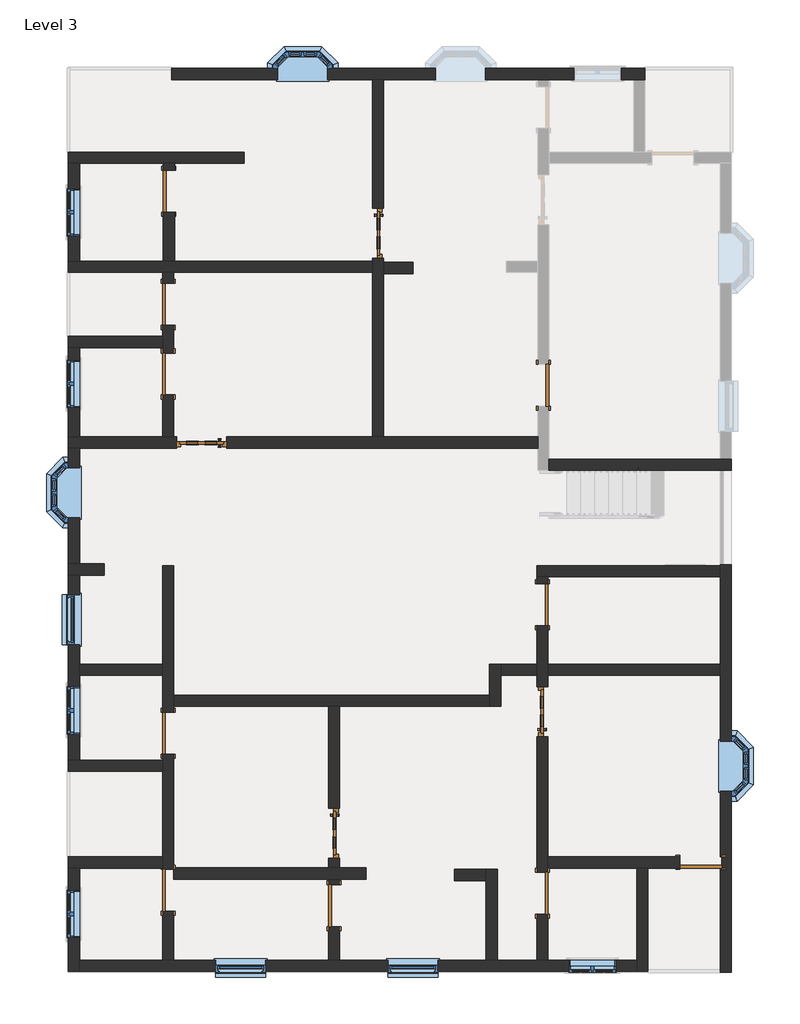
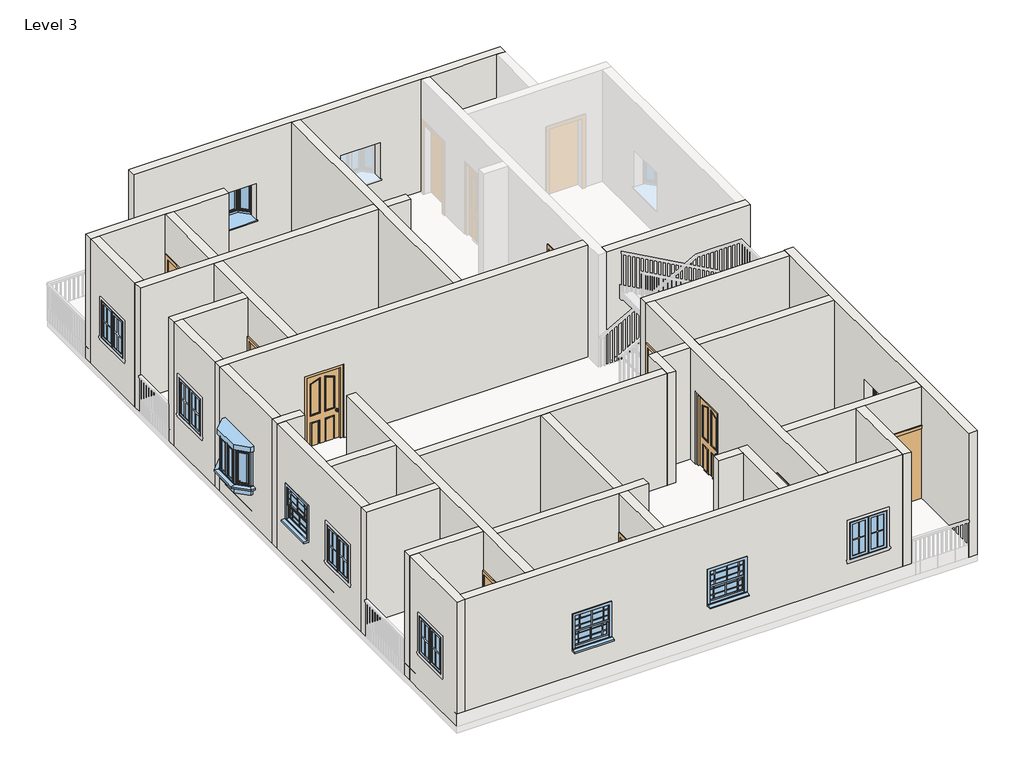
# One storey, part 1 of 4: 34 walls, 14 doors, 11 windows.
"""IFC4 building model written with IfcOpenShell, lengths in millimetres."""

from ifc_helpers import new_model, si_unit, frame, origin, place, context, project, spatial, polyline, outline, extrude, faceted_brep, transform, mapped, element, save
from components import doors_extsgl_12_910x2110mm_9a09825e, door_fadea3f2, door_53b1b562, window_910x910mm_67ef725a, window_c29befe5, windows_sash_w_bars_1_910x910mm_b688f793

model = new_model("IFC4")

# Units and contexts
model_context = context("Model", 3, world=origin())
ifc_project = project(units=[si_unit("LENGTHUNIT", "METRE", prefix="MILLI")], contexts=[model_context])

# Site, building, storey
site = spatial("IfcSite", under=ifc_project)
building = spatial("IfcBuilding", under=site)
storey = spatial("IfcBuildingStorey", under=building, Name="Level 3", Elevation=6096.0)

# Doors
placement = place(None, origin())
doors_extsgl_12_910x2110mm_shape = doors_extsgl_12_910x2110mm_9a09825e(model_context)
element("IfcDoor", 1, ObjectType="Doors_ExtSgl_12 : 910x2110mm", at=placement, inside=storey, context=model_context, shape_type="MappedRepresentation", body=[
    mapped(doors_extsgl_12_910x2110mm_shape, transform((-1409.2058717, 5320.2339901, 6096.0), x_axis=(0.0, -1.0, 0.0), y_axis=(1.0, 0.0, 0.0), z_axis=(0.0, 0.0, 1.0))),
])
element("IfcDoor", 2, ObjectType="Doors_ExtSgl_12 : 910x2110mm", at=placement, inside=storey, context=model_context, shape_type="MappedRepresentation", body=[
    mapped(doors_extsgl_12_910x2110mm_shape, transform((-4622.3058717, 1514.4547293, 6096.0), x_axis=(-1.0, 0.0, 0.0), y_axis=(0.0, -1.0, 0.0), z_axis=(0.0, 0.0, 1.0))),
])
element("IfcDoor", 3, ObjectType="Doors_ExtSgl_12 : 910x2110mm", at=placement, inside=storey, context=model_context, shape_type="MappedRepresentation", body=[
    mapped(doors_extsgl_12_910x2110mm_shape, transform((-2209.3058717, -5597.5452707, 6096.0), x_axis=(0.0, -1.0, 0.0), y_axis=(1.0, 0.0, 0.0), z_axis=(0.0, 0.0, 1.0))),
])
element("IfcDoor", 4, ObjectType="Doors_ExtSgl_12 : 910x2110mm", at=placement, inside=storey, context=model_context, shape_type="MappedRepresentation", body=[
    mapped(doors_extsgl_12_910x2110mm_shape, transform((1587.9941283, -3384.0437545, 6096.0), x_axis=(0.0, 1.0, 0.0), y_axis=(-1.0, 0.0, 0.0), z_axis=(0.0, 0.0, 1.0))),
])
door_shape = door_fadea3f2(model_context)
element("IfcDoor", 5, ObjectType="Single-Flush : 30\" x 80\"", at=placement, inside=storey, context=model_context, shape_type="MappedRepresentation", body=[
    mapped(door_shape, transform((-5219.2058717, 6086.4547293, 6096.0), x_axis=(0.0, 1.0, 0.0), y_axis=(-1.0, 0.0, 0.0), z_axis=(0.0, 0.0, 1.0))),
])
element("IfcDoor", 6, ObjectType="Single-Flush : 30\" x 80\"", at=placement, inside=storey, context=model_context, shape_type="MappedRepresentation", body=[
    mapped(door_shape, transform((-5231.9058717, -6637.2703483, 6096.0), x_axis=(0.0, 1.0, 0.0), y_axis=(-1.0, 0.0, 0.0), z_axis=(0.0, 0.0, 1.0))),
])
element("IfcDoor", 7, ObjectType="Single-Flush : 30\" x 80\"", at=placement, inside=storey, context=model_context, shape_type="MappedRepresentation", body=[
    mapped(door_shape, transform((-2209.3058717, -6918.3452707, 6096.0), x_axis=(0.0, 1.0, 0.0), y_axis=(-1.0, 0.0, 0.0), z_axis=(0.0, 0.0, 1.0))),
])
door_2_shape = door_53b1b562(model_context)
element("IfcDoor", 8, ObjectType="Single-Flush : 30\" x 80\"", at=placement, inside=storey, context=model_context, shape_type="MappedRepresentation", body=[
    mapped(door_2_shape, transform((-5231.9058717, 2759.0547293, 6096.0), x_axis=(0.0, -1.0, 0.0), y_axis=(1.0, 0.0, 0.0), z_axis=(0.0, 0.0, 1.0))),
])
element("IfcDoor", 9, ObjectType="Single-Flush : 30\" x 80\"", at=placement, inside=storey, context=model_context, shape_type="MappedRepresentation", body=[
    mapped(door_2_shape, transform((-5231.9058717, -3778.816952, 6096.0), x_axis=(0.0, -1.0, 0.0), y_axis=(1.0, 0.0, 0.0), z_axis=(0.0, 0.0, 1.0))),
])
element("IfcDoor", 10, ObjectType="Single-Flush : 30\" x 80\"", at=placement, inside=storey, context=model_context, shape_type="MappedRepresentation", body=[
    mapped(door_2_shape, transform((1587.9941283, -6689.7452707, 6096.0), x_axis=(0.0, 1.0, 0.0), y_axis=(-1.0, 0.0, 0.0), z_axis=(0.0, 0.0, 1.0))),
])
element("IfcDoor", 11, ObjectType="Single-Flush : 30\" x 80\"", at=placement, inside=storey, context=model_context, shape_type="MappedRepresentation", body=[
    mapped(door_2_shape, transform((4470.8941283, -6130.9452707, 6096.0), x_axis=(1.0, 0.0, 0.0), y_axis=(0.0, 1.0, 0.0), z_axis=(0.0, 0.0, 1.0))),
])
element("IfcDoor", 12, ObjectType="Single-Flush : 30\" x 80\"", at=placement, inside=storey, context=model_context, shape_type="MappedRepresentation", body=[
    mapped(door_2_shape, transform((1587.9941283, -1440.3867138, 6096.0), x_axis=(0.0, 1.0, 0.0), y_axis=(-1.0, 0.0, 0.0), z_axis=(0.0, 0.0, 1.0))),
])
element("IfcDoor", 13, ObjectType="Single-Flush : 30\" x 80\"", at=placement, inside=storey, context=model_context, shape_type="MappedRepresentation", body=[
    mapped(door_2_shape, transform((1600.6941283, 2555.8547293, 6096.0), x_axis=(0.0, 1.0, 0.0), y_axis=(-1.0, 0.0, 0.0), z_axis=(0.0, 0.0, 1.0))),
])
element("IfcDoor", 14, ObjectType="Single-Flush : 30\" x 80\"", at=placement, inside=storey, context=model_context, shape_type="MappedRepresentation", body=[
    mapped(door_2_shape, transform((-5231.9058717, 4026.9443597, 6096.0), x_axis=(0.0, -1.0, 0.0), y_axis=(1.0, 0.0, 0.0), z_axis=(0.0, 0.0, 1.0))),
])

# Walls
element("IfcWall", 15, ObjectType="Generic - 4.5\"", at=placement, inside=storey, context=model_context, shape_type="Brep", body=[
    faceted_brep([(-1510.8058717, 4865.2339901, 8206.0), (-1510.8058717, 4865.2339901, 6096.0), (-1510.8058717, 4812.2339901, 6096.0), (-1510.8058717, 4609.0339901, 6096.0), (-1510.8058717, 1616.0547293, 6096.0), (-1510.8058717, 1616.0547293, 9144.0), (-1510.8058717, 4609.0339901, 9144.0), (-1510.8058717, 4812.2339901, 9144.0), (-1510.8058717, 8118.4547293, 9144.0), (-1510.8058717, 8118.4547293, 6096.0), (-1510.8058717, 5775.2339901, 6096.0), (-1510.8058717, 5775.2339901, 8206.0), (-1307.6058717, 1616.0547293, 6096.0), (-1307.6058717, 4587.8547293, 6096.0), (-1307.6058717, 4791.0547293, 6096.0), (-1307.6058717, 4865.2339901, 6096.0), (-1307.6058717, 4865.2339901, 8206.0), (-1307.6058717, 5775.2339901, 8206.0), (-1307.6058717, 5775.2339901, 6096.0), (-1307.6058717, 8118.4547293, 6096.0), (-1307.6058717, 8118.4547293, 9144.0), (-1307.6058717, 4791.0547293, 9144.0), (-1307.6058717, 4587.8547293, 9144.0), (-1307.6058717, 1616.0547293, 9144.0)], [[[0, 1, 2, 3, 4, 5, 6, 7, 8, 9, 10, 11]], [[12, 13, 14, 15, 16, 17, 18, 19, 20, 21, 22, 23]], [[10, 9, 19, 18]], [[4, 3, 2, 1, 15, 14, 13, 12]], [[8, 7, 6, 5, 23, 22, 21, 20]], [[9, 8, 20, 19]], [[5, 4, 12, 23]], [[18, 17, 11, 10]], [[16, 15, 1, 0]], [[17, 16, 0, 11]]]),
])
element("IfcWall", 16, ObjectType="Generic - 4.5\"", at=placement, inside=storey, context=model_context, shape_type="Brep", body=[
    faceted_brep([(-7048.0058717, 4609.0339901, 6096.0), (-5333.5058717, 4609.0339901, 6096.0), (-5130.3058717, 4609.0339901, 6096.0), (-1510.8058717, 4609.0339901, 6096.0), (-1510.8058717, 4609.0339901, 9144.0), (-5130.3058717, 4609.0339901, 9144.0), (-5333.5058717, 4609.0339901, 9144.0), (-7048.0058717, 4609.0339901, 9144.0), (-7048.0058717, 4812.2339901, 6096.0), (-7048.0058717, 4812.2339901, 9144.0), (-6844.8058717, 4812.2339901, 9144.0), (-5320.8058717, 4812.2339901, 9144.0), (-5117.6058717, 4812.2339901, 9144.0), (-1510.8058717, 4812.2339901, 9144.0), (-1510.8058717, 4812.2339901, 6096.0), (-5117.6058717, 4812.2339901, 6096.0), (-5320.8058717, 4812.2339901, 6096.0), (-6844.8058717, 4812.2339901, 6096.0)], [[[0, 1, 2, 3, 4, 5, 6, 7]], [[8, 9, 10, 11, 12, 13, 14, 15, 16, 17]], [[3, 2, 1, 0, 8, 17, 16, 15, 14]], [[7, 6, 5, 4, 13, 12, 11, 10, 9]], [[4, 3, 14, 13]], [[0, 7, 9, 8]]]),
])
element("IfcWall", 17, ObjectType="Generic - 4.5\"", at=placement, inside=storey, context=model_context, shape_type="Brep", body=[
    faceted_brep([(-5333.5058717, 3645.9443597, 8128.0), (-5333.5058717, 3645.9443597, 6096.0), (-5333.5058717, 3444.8547293, 6096.0), (-5333.5058717, 3241.6547293, 6096.0), (-5333.5058717, 3140.0547293, 6096.0), (-5333.5058717, 3140.0547293, 8128.0), (-5333.5058717, 2378.0547293, 8128.0), (-5333.5058717, 2378.0547293, 6096.0), (-5333.5058717, 1616.0547293, 6096.0), (-5333.5058717, 1616.0547293, 9144.0), (-5333.5058717, 3241.6547293, 9144.0), (-5333.5058717, 3444.8547293, 9144.0), (-5333.5058717, 4609.0339901, 9144.0), (-5333.5058717, 4609.0339901, 6096.0), (-5333.5058717, 4407.9443597, 6096.0), (-5333.5058717, 4407.9443597, 8128.0), (-5130.3058717, 3140.0547293, 6096.0), (-5130.3058717, 3645.9443597, 6096.0), (-5130.3058717, 3645.9443597, 8128.0), (-5130.3058717, 4407.9443597, 8128.0), (-5130.3058717, 4407.9443597, 6096.0), (-5130.3058717, 4609.0339901, 6096.0), (-5130.3058717, 4609.0339901, 9144.0), (-5130.3058717, 1616.0547293, 9144.0), (-5130.3058717, 1616.0547293, 6096.0), (-5130.3058717, 2378.0547293, 6096.0), (-5130.3058717, 2378.0547293, 8128.0), (-5130.3058717, 3140.0547293, 8128.0)], [[[0, 1, 2, 3, 4, 5, 6, 7, 8, 9, 10, 11, 12, 13, 14, 15]], [[16, 17, 18, 19, 20, 21, 22, 23, 24, 25, 26, 27]], [[8, 7, 25, 24]], [[14, 13, 21, 20]], [[4, 3, 2, 1, 17, 16]], [[12, 11, 10, 9, 23, 22]], [[13, 12, 22, 21]], [[9, 8, 24, 23]], [[26, 25, 7, 6]], [[27, 26, 6, 5]], [[16, 27, 5, 4]], [[18, 17, 1, 0]], [[19, 18, 0, 15]], [[20, 19, 15, 14]]]),
])
element("IfcWall", 18, ObjectType="Generic - 4.5\"", at=placement, inside=storey, context=model_context, shape_type="Brep", body=[
    faceted_brep([(-5130.3058717, -6256.2703483, 8128.0), (-5130.3058717, -6256.2703483, 6096.0), (-5130.3058717, -6230.8703483, 6096.0), (-5130.3058717, -4159.816952, 6096.0), (-5130.3058717, -4159.816952, 8128.0), (-5130.3058717, -3397.816952, 8128.0), (-5130.3058717, -3397.816952, 6096.0), (-5130.3058717, -3286.1452707, 6096.0), (-5130.3058717, -3082.9452707, 6096.0), (-5130.3058717, -733.4452707, 6096.0), (-5130.3058717, -733.4452707, 9144.0), (-5130.3058717, -3082.9452707, 9144.0), (-5130.3058717, -3286.1452707, 9144.0), (-5130.3058717, -6230.8703483, 9144.0), (-5130.3058717, -6434.0703483, 9144.0), (-5130.3058717, -7908.9452707, 9144.0), (-5130.3058717, -7908.9452707, 6096.0), (-5130.3058717, -7018.2703483, 6096.0), (-5130.3058717, -7018.2703483, 8128.0), (-5333.5058717, -4159.816952, 6096.0), (-5333.5058717, -4271.4886333, 6096.0), (-5333.5058717, -4474.6886333, 6096.0), (-5333.5058717, -6029.3452707, 6096.0), (-5333.5058717, -6232.5452707, 6096.0), (-5333.5058717, -6256.2703483, 6096.0), (-5333.5058717, -6256.2703483, 8128.0), (-5333.5058717, -7018.2703483, 8128.0), (-5333.5058717, -7018.2703483, 6096.0), (-5333.5058717, -7908.9452707, 6096.0), (-5333.5058717, -7908.9452707, 9144.0), (-5333.5058717, -6232.5452707, 9144.0), (-5333.5058717, -6029.3452707, 9144.0), (-5333.5058717, -4474.6886333, 9144.0), (-5333.5058717, -4271.4886333, 9144.0), (-5333.5058717, -2727.3452707, 9144.0), (-5333.5058717, -2524.1452707, 9144.0), (-5333.5058717, -733.4452707, 9144.0), (-5333.5058717, -733.4452707, 6096.0), (-5333.5058717, -2524.1452707, 6096.0), (-5333.5058717, -2727.3452707, 6096.0), (-5333.5058717, -3397.816952, 6096.0), (-5333.5058717, -3397.816952, 8128.0), (-5333.5058717, -4159.816952, 8128.0)], [[[0, 1, 2, 3, 4, 5, 6, 7, 8, 9, 10, 11, 12, 13, 14, 15, 16, 17, 18]], [[19, 20, 21, 22, 23, 24, 25, 26, 27, 28, 29, 30, 31, 32, 33, 34, 35, 36, 37, 38, 39, 40, 41, 42]], [[40, 39, 38, 37, 9, 8, 7, 6]], [[17, 16, 28, 27]], [[3, 2, 1, 24, 23, 22, 21, 20, 19]], [[10, 9, 37, 36]], [[15, 14, 13, 12, 11, 10, 36, 35, 34, 33, 32, 31, 30, 29]], [[4, 3, 19, 42]], [[5, 4, 42, 41]], [[6, 5, 41, 40]], [[25, 24, 1, 0]], [[26, 25, 0, 18]], [[27, 26, 18, 17]], [[16, 15, 29, 28]]]),
])
element("IfcWall", 19, ObjectType="Generic - 4.5\"", at=placement, inside=storey, context=model_context, shape_type="Brep", body=[
    faceted_brep([(-7048.0058717, -898.5452707, 6096.0), (-6844.8058717, -898.5452707, 6096.0), (-6400.7404065, -898.5452707, 6096.0), (-6400.7404065, -898.5452707, 9144.0), (-6844.8058717, -898.5452707, 9144.0), (-7048.0058717, -898.5452707, 9144.0), (-7048.0058717, -695.3452707, 6096.0), (-7048.0058717, -695.3452707, 9144.0), (-6844.8058717, -695.3452707, 9144.0), (-6400.7404065, -695.3452707, 9144.0), (-6400.7404065, -695.3452707, 6096.0), (-6844.8058717, -695.3452707, 6096.0)], [[[0, 1, 2, 3, 4, 5]], [[6, 7, 8, 9, 10, 11]], [[2, 1, 0, 6, 11, 10]], [[3, 2, 10, 9]], [[5, 4, 3, 9, 8, 7]], [[0, 5, 7, 6]]]),
])
element("IfcWall", 20, ObjectType="Generic - 4.5\"", at=placement, inside=storey, context=model_context, shape_type="Brep", body=[
    faceted_brep([(-7048.0058717, 6594.4547293, 6096.0), (-6844.8058717, 6594.4547293, 6096.0), (-5320.8058717, 6594.4547293, 6096.0), (-5117.6058717, 6594.4547293, 6096.0), (-3847.6058717, 6594.4547293, 6096.0), (-3847.6058717, 6594.4547293, 9144.0), (-5117.6058717, 6594.4547293, 9144.0), (-5320.8058717, 6594.4547293, 9144.0), (-6844.8058717, 6594.4547293, 9144.0), (-7048.0058717, 6594.4547293, 9144.0), (-7048.0058717, 6797.6547293, 6096.0), (-7048.0058717, 6797.6547293, 9144.0), (-3847.6058717, 6797.6547293, 9144.0), (-3847.6058717, 6797.6547293, 6096.0)], [[[0, 1, 2, 3, 4, 5, 6, 7, 8, 9]], [[10, 11, 12, 13]], [[4, 3, 2, 1, 0, 10, 13]], [[5, 4, 13, 12]], [[9, 8, 7, 6, 5, 12, 11]], [[0, 9, 11, 10]]]),
])
element("IfcWall", 21, ObjectType="Generic - 4.5\"", at=placement, inside=storey, context=model_context, shape_type="Brep", body=[
    faceted_brep([(-7048.0058717, 3241.6547293, 6096.0), (-6844.8058717, 3241.6547293, 6096.0), (-5333.5058717, 3241.6547293, 6096.0), (-5333.5058717, 3241.6547293, 9144.0), (-6844.8058717, 3241.6547293, 9144.0), (-7048.0058717, 3241.6547293, 9144.0), (-7048.0058717, 3444.8547293, 6096.0), (-7048.0058717, 3444.8547293, 9144.0), (-5333.5058717, 3444.8547293, 9144.0), (-5333.5058717, 3444.8547293, 6096.0)], [[[0, 1, 2, 3, 4, 5]], [[6, 7, 8, 9]], [[2, 1, 0, 6, 9]], [[5, 4, 3, 8, 7]], [[3, 2, 9, 8]], [[0, 5, 7, 6]]]),
])
element("IfcWall", 22, ObjectType="Generic - 4.5\"", at=placement, inside=storey, context=model_context, shape_type="Brep", body=[
    faceted_brep([(-7048.0058717, 1412.8547293, 6096.0), (-6844.8058717, 1412.8547293, 6096.0), (-5077.3058717, 1412.8547293, 6096.0), (-5077.3058717, 1412.8547293, 8206.0), (-4167.3058717, 1412.8547293, 8206.0), (-4167.3058717, 1412.8547293, 6096.0), (1499.0941283, 1412.8547293, 6096.0), (1499.0941283, 1412.8547293, 9144.0), (-6844.8058717, 1412.8547293, 9144.0), (-7048.0058717, 1412.8547293, 9144.0), (-5077.3058717, 1616.0547293, 8206.0), (-5077.3058717, 1616.0547293, 6096.0), (-5130.3058717, 1616.0547293, 6096.0), (-5333.5058717, 1616.0547293, 6096.0), (-6844.8058717, 1616.0547293, 6096.0), (-7048.0058717, 1616.0547293, 6096.0), (-7048.0058717, 1616.0547293, 9144.0), (-6844.8058717, 1616.0547293, 9144.0), (-5333.5058717, 1616.0547293, 9144.0), (-5130.3058717, 1616.0547293, 9144.0), (-1510.8058717, 1616.0547293, 9144.0), (-1307.6058717, 1616.0547293, 9144.0), (1499.0941283, 1616.0547293, 9144.0), (1499.0941283, 1616.0547293, 6096.0), (-1307.6058717, 1616.0547293, 6096.0), (-1510.8058717, 1616.0547293, 6096.0), (-4167.3058717, 1616.0547293, 6096.0), (-4167.3058717, 1616.0547293, 8206.0)], [[[0, 1, 2, 3, 4, 5, 6, 7, 8, 9]], [[10, 11, 12, 13, 14, 15, 16, 17, 18, 19, 20, 21, 22, 23, 24, 25, 26, 27]], [[26, 25, 24, 23, 6, 5]], [[15, 14, 13, 12, 11, 2, 1, 0]], [[9, 8, 7, 22, 21, 20, 19, 18, 17, 16]], [[7, 6, 23, 22]], [[5, 4, 27, 26]], [[3, 2, 11, 10]], [[4, 3, 10, 27]], [[0, 9, 16, 15]]]),
])
element("IfcWall", 23, ObjectType="Generic - 4.5\"", at=placement, inside=storey, context=model_context, shape_type="Brep", body=[
    faceted_brep([(1702.2941283, 1006.4547293, 6096.0), (5029.6941283, 1006.4547293, 6096.0), (5029.6941283, 1006.4547293, 9144.0), (1702.2941283, 1006.4547293, 9144.0), (1702.2941283, 1209.6547293, 6096.0), (1702.2941283, 1209.6547293, 9144.0), (4826.4941283, 1209.6547293, 9144.0), (5029.6941283, 1209.6547293, 9144.0), (5029.6941283, 1209.6547293, 6096.0), (4826.4941283, 1209.6547293, 6096.0)], [[[0, 1, 2, 3]], [[4, 5, 6, 7, 8, 9]], [[1, 0, 4, 9, 8]], [[3, 2, 7, 6, 5]], [[0, 3, 5, 4]], [[2, 1, 8, 7]]]),
])
element("IfcWall", 24, ObjectType="Generic - 4.5\"", at=placement, inside=storey, context=model_context, shape_type="Brep", body=[
    faceted_brep([(1486.3941283, -932.3867138, 6096.0), (1689.5941283, -932.3867138, 6096.0), (4826.4941283, -932.3867138, 6096.0), (4826.4941283, -932.3867138, 9144.0), (1689.5941283, -932.3867138, 9144.0), (1486.3941283, -932.3867138, 9144.0), (1486.3941283, -729.1867138, 6096.0), (1486.3941283, -729.1867138, 9144.0), (4826.4941283, -729.1867138, 9144.0), (4826.4941283, -729.1867138, 6096.0)], [[[0, 1, 2, 3, 4, 5]], [[6, 7, 8, 9]], [[2, 1, 0, 6, 9]], [[5, 4, 3, 8, 7]], [[3, 2, 9, 8]], [[0, 5, 7, 6]]]),
])
element("IfcWall", 25, ObjectType="Generic - 4.5\"", at=placement, inside=storey, context=model_context, shape_type="Brep", body=[
    faceted_brep([(1486.3941283, -932.3867138, 6096.0), (1486.3941283, -1059.3867138, 6096.0), (1486.3941283, -1059.3867138, 8128.0), (1486.3941283, -1821.3867138, 8128.0), (1486.3941283, -1821.3867138, 6096.0), (1486.3941283, -2520.4437545, 6096.0), (1486.3941283, -2723.6437545, 6096.0), (1486.3941283, -2929.0437545, 6096.0), (1486.3941283, -2929.0437545, 8206.0), (1486.3941283, -3839.0437545, 8206.0), (1486.3941283, -3839.0437545, 6096.0), (1486.3941283, -6308.7452707, 6096.0), (1486.3941283, -6308.7452707, 8128.0), (1486.3941283, -7070.7452707, 8128.0), (1486.3941283, -7070.7452707, 6096.0), (1486.3941283, -7908.9452707, 6096.0), (1486.3941283, -7908.9452707, 9144.0), (1486.3941283, -2723.6437545, 9144.0), (1486.3941283, -2520.4437545, 9144.0), (1486.3941283, -932.3867138, 9144.0), (1689.5941283, -1059.3867138, 8128.0), (1689.5941283, -1059.3867138, 6096.0), (1689.5941283, -932.3867138, 6096.0), (1689.5941283, -932.3867138, 9144.0), (1689.5941283, -2520.4437545, 9144.0), (1689.5941283, -2723.6437545, 9144.0), (1689.5941283, -6029.3452707, 9144.0), (1689.5941283, -6232.5452707, 9144.0), (1689.5941283, -7908.9452707, 9144.0), (1689.5941283, -7908.9452707, 6096.0), (1689.5941283, -7070.7452707, 6096.0), (1689.5941283, -7070.7452707, 8128.0), (1689.5941283, -6308.7452707, 8128.0), (1689.5941283, -6308.7452707, 6096.0), (1689.5941283, -6232.5452707, 6096.0), (1689.5941283, -6029.3452707, 6096.0), (1689.5941283, -3839.0437545, 6096.0), (1689.5941283, -3839.0437545, 8206.0), (1689.5941283, -2929.0437545, 8206.0), (1689.5941283, -2929.0437545, 6096.0), (1689.5941283, -2723.6437545, 6096.0), (1689.5941283, -2520.4437545, 6096.0), (1689.5941283, -1821.3867138, 6096.0), (1689.5941283, -1821.3867138, 8128.0)], [[[0, 1, 2, 3, 4, 5, 6, 7, 8, 9, 10, 11, 12, 13, 14, 15, 16, 17, 18, 19]], [[20, 21, 22, 23, 24, 25, 26, 27, 28, 29, 30, 31, 32, 33, 34, 35, 36, 37, 38, 39, 40, 41, 42, 43]], [[30, 29, 15, 14]], [[36, 35, 34, 33, 11, 10]], [[22, 21, 1, 0]], [[42, 41, 40, 39, 7, 6, 5, 4]], [[19, 18, 17, 16, 28, 27, 26, 25, 24, 23]], [[0, 19, 23, 22]], [[10, 9, 37, 36]], [[8, 7, 39, 38]], [[9, 8, 38, 37]], [[12, 11, 33, 32]], [[13, 12, 32, 31]], [[14, 13, 31, 30]], [[2, 1, 21, 20]], [[3, 2, 20, 43]], [[4, 3, 43, 42]], [[16, 15, 29, 28]]]),
])
element("IfcWall", 26, ObjectType="Generic - 4.5\"", at=placement, inside=storey, context=model_context, shape_type="SweptSolid", body=[
    extrude(outline(polyline([(4826.4941283, -2723.6437545), (1689.5941283, -2723.6437545), (1689.5941283, -2520.4437545), (4826.4941283, -2520.4437545), (4826.4941283, -2723.6437545)])), frame((0.0, 0.0, 6096.0), z_axis=(0.0, 0.0, 1.0), x_axis=(1.0, 0.0, 0.0)), (0.0, 0.0, 1.0), 3048.0),
])
element("IfcWall", 27, ObjectType="Generic - 4.5\"", at=placement, inside=storey, context=model_context, shape_type="Brep", body=[
    faceted_brep([(4826.4941283, -6232.5452707, 9144.0), (3505.6941283, -6232.5452707, 9144.0), (3302.4941283, -6232.5452707, 9144.0), (1689.5941283, -6232.5452707, 9144.0), (1689.5941283, -6232.5452707, 6096.0), (3302.4941283, -6232.5452707, 6096.0), (3505.6941283, -6232.5452707, 6096.0), (4089.8941283, -6232.5452707, 6096.0), (4089.8941283, -6232.5452707, 8128.0), (4826.4941283, -6232.5452707, 8128.0), (1689.5941283, -6029.3452707, 9144.0), (4826.4941283, -6029.3452707, 9144.0), (4826.4941283, -6029.3452707, 8128.0), (4089.8941283, -6029.3452707, 8128.0), (4089.8941283, -6029.3452707, 6096.0), (1689.5941283, -6029.3452707, 6096.0)], [[[0, 1, 2, 3, 4, 5, 6, 7, 8, 9]], [[10, 11, 12, 13, 14, 15]], [[4, 15, 14, 7, 6, 5]], [[3, 2, 1, 0, 11, 10]], [[11, 0, 9, 12]], [[4, 3, 10, 15]], [[8, 13, 12, 9]], [[13, 8, 7, 14]]]),
])
element("IfcWall", 28, ObjectType="Generic - 4.5\"", at=placement, inside=storey, context=model_context, shape_type="Brep", body=[
    faceted_brep([(3302.4941283, -6232.5452707, 6096.0), (3302.4941283, -7908.9452707, 6096.0), (3302.4941283, -8112.1452707, 6096.0), (3302.4941283, -8112.1452707, 9144.0), (3302.4941283, -7908.9452707, 9144.0), (3302.4941283, -6232.5452707, 9144.0), (3505.6941283, -6232.5452707, 6096.0), (3505.6941283, -6232.5452707, 9144.0), (3505.6941283, -8112.1452707, 9144.0), (3505.6941283, -8112.1452707, 6096.0)], [[[0, 1, 2, 3, 4, 5]], [[6, 7, 8, 9]], [[2, 1, 0, 6, 9]], [[5, 4, 3, 8, 7]], [[0, 5, 7, 6]], [[3, 2, 9, 8]]]),
])
element("IfcWall", 29, ObjectType="Generic - 4.5\"", at=placement, inside=storey, context=model_context, shape_type="SweptSolid", body=[
    extrude(outline(polyline([(-5333.5058717, -2727.3452707), (-6844.8058717, -2727.3452707), (-6844.8058717, -2524.1452707), (-5333.5058717, -2524.1452707), (-5333.5058717, -2727.3452707)])), frame((0.0, 0.0, 6096.0), z_axis=(0.0, 0.0, 1.0), x_axis=(1.0, 0.0, 0.0)), (0.0, 0.0, 1.0), 3048.0),
])
element("IfcWall", 30, ObjectType="Generic - 4.5\"", at=placement, inside=storey, context=model_context, shape_type="Brep", body=[
    faceted_brep([(-7048.0058717, -4474.6886333, 6096.0), (-5333.5058717, -4474.6886333, 6096.0), (-5333.5058717, -4474.6886333, 9144.0), (-7048.0058717, -4474.6886333, 9144.0), (-7048.0058717, -4271.4886333, 6096.0), (-7048.0058717, -4271.4886333, 9144.0), (-6844.8058717, -4271.4886333, 9144.0), (-5333.5058717, -4271.4886333, 9144.0), (-5333.5058717, -4271.4886333, 6096.0), (-6844.8058717, -4271.4886333, 6096.0)], [[[0, 1, 2, 3]], [[4, 5, 6, 7, 8, 9]], [[1, 0, 4, 9, 8]], [[3, 2, 7, 6, 5]], [[2, 1, 8, 7]], [[0, 3, 5, 4]]]),
])
element("IfcWall", 31, ObjectType="Generic - 4.5\"", at=placement, inside=storey, context=model_context, shape_type="Brep", body=[
    faceted_brep([(-7048.0058717, -6232.5452707, 6096.0), (-6844.8058717, -6232.5452707, 6096.0), (-5333.5058717, -6232.5452707, 6096.0), (-5333.5058717, -6232.5452707, 9144.0), (-6844.8058717, -6232.5452707, 9144.0), (-7048.0058717, -6232.5452707, 9144.0), (-7048.0058717, -6029.3452707, 6096.0), (-7048.0058717, -6029.3452707, 9144.0), (-5333.5058717, -6029.3452707, 9144.0), (-5333.5058717, -6029.3452707, 6096.0)], [[[0, 1, 2, 3, 4, 5]], [[6, 7, 8, 9]], [[2, 1, 0, 6, 9]], [[5, 4, 3, 8, 7]], [[3, 2, 9, 8]], [[0, 5, 7, 6]]]),
])
element("IfcWall", 32, ObjectType="Generic - 4.5\"", at=placement, inside=storey, context=model_context, shape_type="Brep", body=[
    faceted_brep([(-5130.3058717, -6434.0703483, 6096.0), (-2310.9058717, -6434.0703483, 6096.0), (-2107.7058717, -6434.0703483, 6096.0), (-1625.1058717, -6434.0703483, 6096.0), (-1625.1058717, -6434.0703483, 9144.0), (-2107.7058717, -6434.0703483, 9144.0), (-2310.9058717, -6434.0703483, 9144.0), (-5130.3058717, -6434.0703483, 9144.0), (-5130.3058717, -6230.8703483, 6096.0), (-5130.3058717, -6230.8703483, 9144.0), (-2310.9058717, -6230.8703483, 9144.0), (-2107.7058717, -6230.8703483, 9144.0), (-1625.1058717, -6230.8703483, 9144.0), (-1625.1058717, -6230.8703483, 6096.0), (-2107.7058717, -6230.8703483, 6096.0), (-2310.9058717, -6230.8703483, 6096.0), (-5130.3058717, -6256.2703483, 6096.0)], [[[0, 1, 2, 3, 4, 5, 6, 7]], [[8, 9, 10, 11, 12, 13, 14, 15]], [[3, 2, 1, 0, 16, 8, 15, 14, 13]], [[4, 3, 13, 12]], [[7, 6, 5, 4, 12, 11, 10, 9]], [[0, 7, 9, 8, 16]]]),
])
element("IfcWall", 33, ObjectType="Generic - 4.5\"", at=placement, inside=storey, context=model_context, shape_type="Brep", body=[
    faceted_brep([(762.4941283, -7908.9452707, 6096.0), (762.4941283, -6257.9452707, 6096.0), (762.4941283, -6257.9452707, 9144.0), (762.4941283, -7908.9452707, 9144.0), (559.2941283, -7908.9452707, 6096.0), (559.2941283, -7908.9452707, 9144.0), (559.2941283, -6461.1452707, 9144.0), (559.2941283, -6257.9452707, 9144.0), (559.2941283, -6257.9452707, 6096.0), (559.2941283, -6461.1452707, 6096.0)], [[[0, 1, 2, 3]], [[4, 5, 6, 7, 8, 9]], [[1, 0, 4, 9, 8]], [[3, 2, 7, 6, 5]], [[2, 1, 8, 7]], [[0, 3, 5, 4]]]),
])
element("IfcWall", 34, ObjectType="Generic - 4.5\"", at=placement, inside=storey, context=model_context, shape_type="SweptSolid", body=[
    extrude(outline(polyline([(-12.2058717, -6257.9452707), (559.2941283, -6257.9452707), (559.2941283, -6461.1452707), (-12.2058717, -6461.1452707), (-12.2058717, -6257.9452707)])), frame((0.0, 0.0, 6096.0), z_axis=(0.0, 0.0, 1.0), x_axis=(1.0, 0.0, 0.0)), (0.0, 0.0, 1.0), 3048.0),
])
element("IfcWall", 35, ObjectType="Generic - 4.5\"", at=placement, inside=storey, context=model_context, shape_type="SweptSolid", body=[
    extrude(outline(polyline([(-3286.1452707, 9144.0), (-3286.1452707, 6096.0), (-5142.5452707, 6096.0), (-5142.5452707, 8206.0), (-6052.5452707, 8206.0), (-6052.5452707, 6096.0), (-6230.8703483, 6096.0), (-6230.8703483, 9144.0), (-3286.1452707, 9144.0)])), frame((-2310.9058717, 0.0, 0.0), z_axis=(1.0, 0.0, 0.0), x_axis=(0.0, 1.0, 0.0)), (0.0, 0.0, 1.0), 203.2),
    extrude(outline(polyline([(-6537.3452707, 6096.0), (-6537.3452707, 8128.0), (-7299.3452707, 8128.0), (-7299.3452707, 6096.0), (-7908.9452707, 6096.0), (-7908.9452707, 9144.0), (-6434.0703483, 9144.0), (-6434.0703483, 6096.0), (-6537.3452707, 6096.0)])), frame((-2310.9058717, 0.0, 0.0), z_axis=(1.0, 0.0, 0.0), x_axis=(0.0, 1.0, 0.0)), (0.0, 0.0, 1.0), 203.2),
])
element("IfcWall", 36, ObjectType="Generic - 4.5\"", at=placement, inside=storey, context=model_context, shape_type="Brep", body=[
    faceted_brep([(-5130.3058717, -3286.1452707, 6096.0), (-2310.9058717, -3286.1452707, 6096.0), (-2107.7058717, -3286.1452707, 6096.0), (622.0199378, -3286.1452707, 6096.0), (622.0199378, -3286.1452707, 9144.0), (-2107.7058717, -3286.1452707, 9144.0), (-2310.9058717, -3286.1452707, 9144.0), (-5130.3058717, -3286.1452707, 9144.0), (-5130.3058717, -3082.9452707, 6096.0), (-5130.3058717, -3082.9452707, 9144.0), (622.0199378, -3082.9452707, 9144.0), (622.0199378, -3082.9452707, 6096.0)], [[[0, 1, 2, 3, 4, 5, 6, 7]], [[8, 9, 10, 11]], [[3, 2, 1, 0, 8, 11]], [[7, 6, 5, 4, 10, 9]], [[0, 7, 9, 8]], [[4, 3, 11, 10]]]),
])
element("IfcWall", 37, ObjectType="Generic - 4.5\"", at=placement, inside=storey, context=model_context, shape_type="Brep", body=[
    faceted_brep([(825.2199378, -3286.1452707, 6096.0), (825.2199378, -2723.6437545, 6096.0), (825.2199378, -2520.4437545, 6096.0), (825.2199378, -2520.4437545, 9144.0), (825.2199378, -2723.6437545, 9144.0), (825.2199378, -3286.1452707, 9144.0), (622.0199378, -3286.1452707, 6096.0), (622.0199378, -3286.1452707, 9144.0), (622.0199378, -3082.9452707, 9144.0), (622.0199378, -2520.4437545, 9144.0), (622.0199378, -2520.4437545, 6096.0), (622.0199378, -3082.9452707, 6096.0)], [[[0, 1, 2, 3, 4, 5]], [[6, 7, 8, 9, 10, 11]], [[2, 1, 0, 6, 11, 10]], [[5, 4, 3, 9, 8, 7]], [[0, 5, 7, 6]], [[3, 2, 10, 9]]]),
])
element("IfcWall", 38, ObjectType="Generic - 4.5\"", at=placement, inside=storey, context=model_context, shape_type="SweptSolid", body=[
    extrude(outline(polyline([(1486.3941283, -2723.6437545), (825.2199378, -2723.6437545), (825.2199378, -2520.4437545), (1486.3941283, -2520.4437545), (1486.3941283, -2723.6437545)])), frame((0.0, 0.0, 6096.0), z_axis=(0.0, 0.0, 1.0), x_axis=(1.0, 0.0, 0.0)), (0.0, 0.0, 1.0), 3048.0),
])
element("IfcWall", 39, ObjectType="Generic - 4.5\"", at=placement, inside=storey, context=model_context, shape_type="SweptSolid", body=[
    extrude(outline(polyline([(-774.2058717, 4587.8547293), (-1307.6058717, 4587.8547293), (-1307.6058717, 4791.0547293), (-774.2058717, 4791.0547293), (-774.2058717, 4587.8547293)])), frame((0.0, 0.0, 6096.0), z_axis=(0.0, 0.0, 1.0), x_axis=(1.0, 0.0, 0.0)), (0.0, 0.0, 1.0), 3048.0),
])
element("IfcWall", 40, ObjectType="Generic - 4.5\"", at=placement, inside=storey, context=model_context, shape_type="SweptSolid", body=[
    extrude(outline(polyline([(6594.4547293, 6096.0), (6467.4547293, 6096.0), (6467.4547293, 8128.0), (5705.4547293, 8128.0), (5705.4547293, 6096.0), (4812.2339901, 6096.0), (4812.2339901, 9144.0), (6594.4547293, 9144.0), (6594.4547293, 6096.0)])), frame((-5320.8058717, 0.0, 0.0), z_axis=(1.0, 0.0, 0.0), x_axis=(0.0, 1.0, 0.0)), (0.0, 0.0, 1.0), 203.2),
])
element("IfcWall", 41, ObjectType="Generic - 9\"", at=placement, inside=storey, context=model_context, shape_type="Brep", body=[
    faceted_brep([(-5168.4058717, 8118.4547293, 6096.0), (-1510.8058717, 8118.4547293, 6096.0), (-1307.6058717, 8118.4547293, 6096.0), (1499.0941283, 8118.4547293, 6096.0), (1702.2941283, 8118.4547293, 6096.0), (3251.6941283, 8118.4547293, 6096.0), (3454.8941283, 8118.4547293, 6096.0), (3454.8941283, 8118.4547293, 9144.0), (3251.6941283, 8118.4547293, 9144.0), (1702.2941283, 8118.4547293, 9144.0), (1499.0941283, 8118.4547293, 9144.0), (-1307.6058717, 8118.4547293, 9144.0), (-1510.8058717, 8118.4547293, 9144.0), (-5168.4058717, 8118.4547293, 9144.0), (-359.2558717, 8118.4547293, 7920.4), (550.7441283, 8118.4547293, 7920.4), (550.7441283, 8118.4547293, 7010.4), (-359.2558717, 8118.4547293, 7010.4), (-3235.8058717, 8118.4547293, 7920.4), (-2325.8058717, 8118.4547293, 7920.4), (-2325.8058717, 8118.4547293, 7010.4), (-3235.8058717, 8118.4547293, 7010.4), (3023.0941283, 8118.4547293, 7924.8), (3023.0941283, 8118.4547293, 7010.4), (2159.4941283, 8118.4547293, 7010.4), (2159.4941283, 8118.4547293, 7924.8), (-5168.4058717, 8321.6547293, 6096.0), (-5168.4058717, 8321.6547293, 9144.0), (3454.8941283, 8321.6547293, 9144.0), (3454.8941283, 8321.6547293, 6096.0), (-359.2558717, 8321.6547293, 7920.4), (-359.2558717, 8321.6547293, 7010.4), (550.7441283, 8321.6547293, 7010.4), (550.7441283, 8321.6547293, 7920.4), (-3235.8058717, 8321.6547293, 7920.4), (-3235.8058717, 8321.6547293, 7010.4), (-2325.8058717, 8321.6547293, 7010.4), (-2325.8058717, 8321.6547293, 7920.4), (3023.0941283, 8321.6547293, 7924.8), (2159.4941283, 8321.6547293, 7924.8), (2159.4941283, 8321.6547293, 7010.4), (3023.0941283, 8321.6547293, 7010.4)], [[[0, 1, 2, 3, 4, 5, 6, 7, 8, 9, 10, 11, 12, 13], [14, 15, 16, 17], [18, 19, 20, 21], [22, 23, 24, 25]], [[26, 27, 28, 29], [30, 31, 32, 33], [34, 35, 36, 37], [38, 39, 40, 41]], [[6, 5, 4, 3, 2, 1, 0, 26, 29]], [[13, 12, 11, 10, 9, 8, 7, 28, 27]], [[0, 13, 27, 26]], [[31, 30, 14, 17]], [[32, 31, 17, 16]], [[33, 32, 16, 15]], [[30, 33, 15, 14]], [[35, 34, 18, 21]], [[36, 35, 21, 20]], [[37, 36, 20, 19]], [[34, 37, 19, 18]], [[23, 22, 38, 41]], [[24, 23, 41, 40]], [[25, 24, 40, 39]], [[22, 25, 39, 38]], [[7, 6, 29, 28]]]),
])
element("IfcWall", 42, ObjectType="Generic - 9\"", at=placement, inside=storey, context=model_context, shape_type="Brep", body=[
    faceted_brep([(4826.4941283, -8124.8452707, 6096.0), (4826.4941283, -8124.8452707, 9144.0), (4826.4941283, -6232.5452707, 9144.0), (4826.4941283, -6029.3452707, 9144.0), (4826.4941283, -2723.6437545, 9144.0), (4826.4941283, -2520.4437545, 9144.0), (4826.4941283, -932.3867138, 9144.0), (4826.4941283, -729.1867138, 9144.0), (4826.4941283, -714.2964201, 9144.0), (4826.4941283, -714.2964201, 6096.0), (4826.4941283, -729.1867138, 6096.0), (4826.4941283, -932.3867138, 6096.0), (4826.4941283, -2520.4437545, 6096.0), (4826.4941283, -2723.6437545, 6096.0), (4826.4941283, -6029.3452707, 6096.0), (4826.4941283, -6029.3452707, 8128.0), (4826.4941283, -6232.5452707, 8128.0), (4826.4941283, -6232.5452707, 6096.0), (4826.4941283, -3921.4945126, 7920.4), (4826.4941283, -4831.4945126, 7920.4), (4826.4941283, -4831.4945126, 7010.4), (4826.4941283, -3921.4945126, 7010.4), (5029.6941283, -8124.8452707, 6096.0), (5029.6941283, -714.2964201, 6096.0), (5029.6941283, -714.2964201, 9144.0), (5029.6941283, -8124.8452707, 9144.0), (5029.6941283, -3921.4945126, 7920.4), (5029.6941283, -3921.4945126, 7010.4), (5029.6941283, -4831.4945126, 7010.4), (5029.6941283, -4831.4945126, 7920.4), (4851.8941283, -6232.5452707, 6096.0), (4851.8941283, -6029.3452707, 6096.0), (4851.8941283, -6232.5452707, 8128.0), (4851.8941283, -6029.3452707, 8128.0)], [[[0, 1, 2, 3, 4, 5, 6, 7, 8, 9, 10, 11, 12, 13, 14, 15, 16, 17], [18, 19, 20, 21]], [[22, 23, 24, 25], [26, 27, 28, 29]], [[23, 22, 0, 17, 30, 31, 14, 13, 12, 11, 10, 9]], [[1, 0, 22, 25]], [[8, 7, 6, 5, 4, 3, 2, 1, 25, 24]], [[9, 8, 24, 23]], [[32, 30, 17, 16]], [[31, 33, 15, 14]], [[33, 32, 16, 15]], [[30, 32, 33, 31]], [[27, 26, 18, 21]], [[28, 27, 21, 20]], [[29, 28, 20, 19]], [[26, 29, 19, 18]]]),
])
element("IfcWall", 43, ObjectType="Generic - 9\"", at=placement, inside=storey, context=model_context, shape_type="SweptSolid", body=[
    extrude(outline(polyline([(6594.4547293, 6096.0), (4812.2339901, 6096.0), (4812.2339901, 9144.0), (6594.4547293, 9144.0), (6594.4547293, 6096.0)]), holes=[polyline([(6135.1443597, 7924.8), (5271.5443597, 7924.8), (5271.5443597, 7010.4), (6135.1443597, 7010.4), (6135.1443597, 7924.8)])]), frame((-7048.0058717, 0.0, 0.0), z_axis=(1.0, 0.0, 0.0), x_axis=(0.0, 1.0, 0.0)), (0.0, 0.0, 1.0), 203.2),
])
element("IfcWall", 44, ObjectType="Generic - 9\"", at=placement, inside=storey, context=model_context, shape_type="SweptSolid", body=[
    extrude(outline(polyline([(3241.6547293, 6096.0), (1616.0547293, 6096.0), (1616.0547293, 9144.0), (3241.6547293, 9144.0), (3241.6547293, 6096.0)]), holes=[polyline([(3013.0547293, 7924.8), (2149.4547293, 7924.8), (2149.4547293, 7010.4), (3013.0547293, 7010.4), (3013.0547293, 7924.8)])]), frame((-7048.0058717, 0.0, 0.0), z_axis=(1.0, 0.0, 0.0), x_axis=(0.0, 1.0, 0.0)), (0.0, 0.0, 1.0), 203.2),
])
element("IfcWall", 45, ObjectType="Generic - 9\"", at=placement, inside=storey, context=model_context, shape_type="Brep", body=[
    faceted_brep([(-7048.0058717, -898.5452707, 6096.0), (-7048.0058717, -4271.4886333, 6096.0), (-7048.0058717, -4271.4886333, 9144.0), (-7048.0058717, -898.5452707, 9144.0), (-7048.0058717, -2166.3452707, 7010.4), (-7048.0058717, -1256.3452707, 7010.4), (-7048.0058717, -1256.3452707, 7920.4), (-7048.0058717, -2166.3452707, 7920.4), (-7048.0058717, -2930.5452707, 7924.8), (-7048.0058717, -3794.1452707, 7924.8), (-7048.0058717, -3794.1452707, 7010.4), (-7048.0058717, -2930.5452707, 7010.4), (-6844.8058717, -898.5452707, 6096.0), (-6844.8058717, -898.5452707, 9144.0), (-6844.8058717, -2524.1452707, 9144.0), (-6844.8058717, -2727.3452707, 9144.0), (-6844.8058717, -4271.4886333, 9144.0), (-6844.8058717, -4271.4886333, 6096.0), (-6844.8058717, -2727.3452707, 6096.0), (-6844.8058717, -2524.1452707, 6096.0), (-6844.8058717, -2166.3452707, 7010.4), (-6844.8058717, -2166.3452707, 7920.4), (-6844.8058717, -1256.3452707, 7920.4), (-6844.8058717, -1256.3452707, 7010.4), (-6844.8058717, -2930.5452707, 7924.8), (-6844.8058717, -2930.5452707, 7010.4), (-6844.8058717, -3794.1452707, 7010.4), (-6844.8058717, -3794.1452707, 7924.8)], [[[0, 1, 2, 3], [4, 5, 6, 7], [8, 9, 10, 11]], [[12, 13, 14, 15, 16, 17, 18, 19], [20, 21, 22, 23], [24, 25, 26, 27]], [[1, 0, 12, 19, 18, 17]], [[3, 2, 16, 15, 14, 13]], [[0, 3, 13, 12]], [[2, 1, 17, 16]], [[21, 20, 4, 7]], [[22, 21, 7, 6]], [[23, 22, 6, 5]], [[20, 23, 5, 4]], [[25, 24, 8, 11]], [[26, 25, 11, 10]], [[27, 26, 10, 9]], [[24, 27, 9, 8]]]),
])
element("IfcWall", 46, ObjectType="Generic - 9\"", at=placement, inside=storey, context=model_context, shape_type="Brep", body=[
    faceted_brep([(-7048.0058717, -6232.5452707, 6096.0), (-7048.0058717, -8112.1452707, 6096.0), (-7048.0058717, -8112.1452707, 9144.0), (-7048.0058717, -6232.5452707, 9144.0), (-7048.0058717, -6638.9452707, 7924.8), (-7048.0058717, -7502.5452707, 7924.8), (-7048.0058717, -7502.5452707, 7010.4), (-7048.0058717, -6638.9452707, 7010.4), (-6844.8058717, -6232.5452707, 6096.0), (-6844.8058717, -6232.5452707, 9144.0), (-6844.8058717, -7908.9452707, 9144.0), (-6844.8058717, -8112.1452707, 9144.0), (-6844.8058717, -8112.1452707, 6096.0), (-6844.8058717, -7908.9452707, 6096.0), (-6844.8058717, -6638.9452707, 7924.8), (-6844.8058717, -6638.9452707, 7010.4), (-6844.8058717, -7502.5452707, 7010.4), (-6844.8058717, -7502.5452707, 7924.8)], [[[0, 1, 2, 3], [4, 5, 6, 7]], [[8, 9, 10, 11, 12, 13], [14, 15, 16, 17]], [[1, 0, 8, 13, 12]], [[3, 2, 11, 10, 9]], [[0, 3, 9, 8]], [[2, 1, 12, 11]], [[15, 14, 4, 7]], [[16, 15, 7, 6]], [[17, 16, 6, 5]], [[14, 17, 5, 4]]]),
])
element("IfcWall", 47, ObjectType="Generic - 9\"", at=placement, inside=storey, context=model_context, shape_type="Brep", body=[
    faceted_brep([(-6844.8058717, -8112.1452707, 6096.0), (3302.4941283, -8112.1452707, 6096.0), (3302.4941283, -8112.1452707, 9144.0), (-6844.8058717, -8112.1452707, 9144.0), (-3456.1058717, -8112.1452707, 7010.4), (-4366.1058717, -8112.1452707, 7010.4), (-4366.1058717, -8112.1452707, 7920.4), (-3456.1058717, -8112.1452707, 7920.4), (-319.2058717, -8112.1452707, 7010.4), (-1229.2058717, -8112.1452707, 7010.4), (-1229.2058717, -8112.1452707, 7920.4), (-319.2058717, -8112.1452707, 7920.4), (2064.2441283, -8112.1452707, 7924.8), (2927.8441283, -8112.1452707, 7924.8), (2927.8441283, -8112.1452707, 7010.4), (2064.2441283, -8112.1452707, 7010.4), (-6844.8058717, -7908.9452707, 6096.0), (-6844.8058717, -7908.9452707, 9144.0), (-5333.5058717, -7908.9452707, 9144.0), (-5130.3058717, -7908.9452707, 9144.0), (-2310.9058717, -7908.9452707, 9144.0), (-2107.7058717, -7908.9452707, 9144.0), (559.2941283, -7908.9452707, 9144.0), (762.4941283, -7908.9452707, 9144.0), (1486.3941283, -7908.9452707, 9144.0), (1689.5941283, -7908.9452707, 9144.0), (3302.4941283, -7908.9452707, 9144.0), (3302.4941283, -7908.9452707, 6096.0), (1689.5941283, -7908.9452707, 6096.0), (1486.3941283, -7908.9452707, 6096.0), (762.4941283, -7908.9452707, 6096.0), (559.2941283, -7908.9452707, 6096.0), (-2107.7058717, -7908.9452707, 6096.0), (-2310.9058717, -7908.9452707, 6096.0), (-5130.3058717, -7908.9452707, 6096.0), (-5333.5058717, -7908.9452707, 6096.0), (-3456.1058717, -7908.9452707, 7010.4), (-3456.1058717, -7908.9452707, 7920.4), (-4366.1058717, -7908.9452707, 7920.4), (-4366.1058717, -7908.9452707, 7010.4), (-319.2058717, -7908.9452707, 7010.4), (-319.2058717, -7908.9452707, 7920.4), (-1229.2058717, -7908.9452707, 7920.4), (-1229.2058717, -7908.9452707, 7010.4), (2064.2441283, -7908.9452707, 7924.8), (2064.2441283, -7908.9452707, 7010.4), (2927.8441283, -7908.9452707, 7010.4), (2927.8441283, -7908.9452707, 7924.8)], [[[0, 1, 2, 3], [4, 5, 6, 7], [8, 9, 10, 11], [12, 13, 14, 15]], [[16, 17, 18, 19, 20, 21, 22, 23, 24, 25, 26, 27, 28, 29, 30, 31, 32, 33, 34, 35], [36, 37, 38, 39], [40, 41, 42, 43], [44, 45, 46, 47]], [[1, 0, 16, 35, 34, 33, 32, 31, 30, 29, 28, 27]], [[3, 2, 26, 25, 24, 23, 22, 21, 20, 19, 18, 17]], [[2, 1, 27, 26]], [[0, 3, 17, 16]], [[37, 36, 4, 7]], [[38, 37, 7, 6]], [[39, 38, 6, 5]], [[36, 39, 5, 4]], [[41, 40, 8, 11]], [[42, 41, 11, 10]], [[43, 42, 10, 9]], [[40, 43, 9, 8]], [[45, 44, 12, 15]], [[46, 45, 15, 14]], [[47, 46, 14, 13]], [[44, 47, 13, 12]]]),
])
element("IfcWall", 48, ObjectType="Generic - 9\"", at=placement, inside=storey, context=model_context, shape_type="SweptSolid", body=[
    extrude(outline(polyline([(1412.8547293, 6096.0), (-695.3452707, 6096.0), (-695.3452707, 9144.0), (1412.8547293, 9144.0), (1412.8547293, 6096.0)]), holes=[polyline([(145.0547293, 7920.4), (145.0547293, 7010.4), (1055.0547293, 7010.4), (1055.0547293, 7920.4), (145.0547293, 7920.4)])]), frame((-7048.0058717, 0.0, 0.0), z_axis=(1.0, 0.0, 0.0), x_axis=(0.0, 1.0, 0.0)), (0.0, 0.0, 1.0), 203.2),
])

# Windows
window_910x910mm_shape = window_910x910mm_67ef725a(model_context)
element("IfcWindow", 49, ObjectType="910x910mm", at=placement, inside=storey, context=model_context, shape_type="MappedRepresentation", body=[
    mapped(window_910x910mm_shape, transform((4919.6375605, -4946.4945126, 5810.4), x_axis=(0.0, -1.0, 0.0), y_axis=(1.0, 0.0, 0.0), z_axis=(0.0, 0.0, 1.0))),
])
element("IfcWindow", 50, ObjectType="910x910mm", at=placement, inside=storey, context=model_context, shape_type="MappedRepresentation", body=[
    mapped(window_910x910mm_shape, transform((-2210.8058717, 8211.5981615, 5810.4), x_axis=(1.0, 0.0, 0.0), y_axis=(0.0, 1.0, 0.0), z_axis=(0.0, 0.0, 1.0))),
])
element("IfcWindow", 51, ObjectType="910x910mm", at=placement, inside=storey, context=model_context, shape_type="MappedRepresentation", body=[
    mapped(window_910x910mm_shape, transform((-6937.9493039, 1170.0547293, 5810.4), x_axis=(0.0, 1.0, 0.0), y_axis=(-1.0, 0.0, 0.0), z_axis=(0.0, 0.0, 1.0))),
])
window_shape = window_c29befe5(model_context)
element("IfcWindow", 52, ObjectType="Window-Casement-Double : 34\" x 36\"", at=placement, inside=storey, context=model_context, shape_type="MappedRepresentation", body=[
    mapped(window_shape, transform((-6946.4058717, 5703.3443597, 6096.0), x_axis=(0.0, 1.0, 0.0), y_axis=(-1.0, 0.0, 0.0), z_axis=(0.0, 0.0, 1.0))),
])
element("IfcWindow", 53, ObjectType="Window-Casement-Double : 34\" x 36\"", at=placement, inside=storey, context=model_context, shape_type="MappedRepresentation", body=[
    mapped(window_shape, transform((-6946.4058717, 2581.2547293, 6096.0), x_axis=(0.0, 1.0, 0.0), y_axis=(-1.0, 0.0, 0.0), z_axis=(0.0, 0.0, 1.0))),
])
element("IfcWindow", 54, ObjectType="Window-Casement-Double : 34\" x 36\"", at=placement, inside=storey, context=model_context, shape_type="MappedRepresentation", body=[
    mapped(window_shape, transform((2496.0441283, -8010.5452707, 6096.0), x_axis=(-1.0, 0.0, 0.0), y_axis=(0.0, -1.0, 0.0), z_axis=(0.0, 0.0, 1.0))),
])
element("IfcWindow", 55, ObjectType="Window-Casement-Double : 34\" x 36\"", at=placement, inside=storey, context=model_context, shape_type="MappedRepresentation", body=[
    mapped(window_shape, transform((-6946.4058717, -7070.7452707, 6096.0), x_axis=(0.0, 1.0, 0.0), y_axis=(-1.0, 0.0, 0.0), z_axis=(0.0, 0.0, 1.0))),
])
element("IfcWindow", 56, ObjectType="Window-Casement-Double : 34\" x 36\"", at=placement, inside=storey, context=model_context, shape_type="MappedRepresentation", body=[
    mapped(window_shape, transform((-6946.4058717, -3362.3452707, 6096.0), x_axis=(0.0, 1.0, 0.0), y_axis=(-1.0, 0.0, 0.0), z_axis=(0.0, 0.0, 1.0))),
])
windows_sash_w_bars_1_910x910mm_shape = windows_sash_w_bars_1_910x910mm_b688f793(model_context)
element("IfcWindow", 57, ObjectType="Windows_Sash_w-Bars_1 : 910x910mm", at=placement, inside=storey, context=model_context, shape_type="MappedRepresentation", body=[
    mapped(windows_sash_w_bars_1_910x910mm_shape, transform((-3911.1058717, -8010.5452707, 6210.4), x_axis=(-1.0, 0.0, 0.0), y_axis=(0.0, -1.0, 0.0), z_axis=(0.0, 0.0, 1.0))),
])
element("IfcWindow", 58, ObjectType="Windows_Sash_w-Bars_1 : 910x910mm", at=placement, inside=storey, context=model_context, shape_type="MappedRepresentation", body=[
    mapped(windows_sash_w_bars_1_910x910mm_shape, transform((-6946.4058717, -1711.3452707, 6210.4), x_axis=(0.0, 1.0, 0.0), y_axis=(-1.0, 0.0, 0.0), z_axis=(0.0, 0.0, 1.0))),
])
element("IfcWindow", 59, ObjectType="Windows_Sash_w-Bars_1 : 910x910mm", at=placement, inside=storey, context=model_context, shape_type="MappedRepresentation", body=[
    mapped(windows_sash_w_bars_1_910x910mm_shape, transform((-774.2058717, -8010.5452707, 6210.4), x_axis=(-1.0, 0.0, 0.0), y_axis=(0.0, -1.0, 0.0), z_axis=(0.0, 0.0, 1.0))),
])

save(model, "model.ifc")

# Revit data of these elements
# Type "Doors_ExtSgl_12 : 910x2110mm"
#   Type Mark = "10"
#   Type Comments = "External Single"
#   Operation = "SingleSwingRight"
#   Construction Type Id = "SGL"
#   Keynote = "L20"
#   Analytic Construction = "Large single-glazed windows"
#   Wrap Layers (Int) from Ext = 0' - 6.98819"
#   Wrap Layers (Ext) from Ext = 0' - 4.03543"
#   Visual Light Transmittance = 0.9
#   Thickness = 0' - 1.73228"
#   Stile Top of Lock rail = 3' - 3.37008"
#   Stile Top Rail = 0' - 5.90551"
#   Stile Shutting = 0' - 4.92126"
#   Stile Muntin Rail = 0' - 4.92126"
#   Stile Lock Rail = 0' - 6.88976"
#   Stile Hanging = 0' - 4.92126"
#   Stile Bottom Rail = 0' - 6.88976"
#   Solar Heat Gain Coefficient = 0.86
#   Rough Width = 2' - 11.82677"
#   Rough Height = 6' - 11.07087"
#   O/A Frame Width = 0' - 2.51969"
#   Heat Transfer Coefficient (U) = 0.979472 BTU/(h·ft²·°F)
#   Handle Z Distance = 3' - 3.37008"
#   Glazing Thickness = 0' - 0.94488"
#   FrameWidth = 0' - 1.65354"
#   FrameOffset - External = 0' - 0.98425"
#   FrameDepth = 0' - 3.50394"
#   Door Panel Width = 2' - 7.77165"
#   Door Panel Thickness = 0' - 1.73228"
#   Door Panel Height = 6' - 6.74016"
#   Cill Thickness = 0' - 2.14567"
#   Cill Projection = 0' - 1.1811"
#   Handle X Distance = 0' - 2.95276"
#   Height = 6' - 11.07087"
#   Structural Tolerance = 0' - 0.25591"
#   Tolerance = 0' - 0.11811"
#   Undercut = 0' - 0.15748"
#   Width = 2' - 11.82677"
#   Cill Extension = 0' - 0.98425"
#   Cavity Closer Width = 0' - 1.9685"
#   Cavity Closer Offset from Ext = 0' - 4.03543"
#   Cavity Closer Depth = 0' - 3.34646"
#   Vis - Ironmongery = yes
#   Vis - Cavity Closers = yes
#   Define Thermal Properties by = 1
#   Function = 1
#   Material Glass = Door - Glazing
#   Material Door = Door - Panel
#   Material Frame = Door - Frame/Mullion
#   Material Ironmongery = Door - Handle
#   Wall Closure = (empty or 0)
# Type "Single-Flush : 30\" x 80\""
#   Type Mark = "5"
#   Construction Type Id = "MDOOR"
#   Assembly Code = "C1020"
#   Analytic Construction = "Metal"
#   Thickness = 0' - 2"
#   Heat Transfer Coefficient (U) = 0.651978 BTU/(h·ft²·°F)
#   Height = 6' - 8"
#   Trim Projection Ext = 0' - 1"
#   Trim Projection Int = 0' - 1"
#   Trim Width = 0' - 3"
#   Width = 2' - 6"
#   Define Thermal Properties by = 1
#   Define Thermal Properties by = 1
#   Door Material = Door - Panel
#   Frame Material = Door - Frame
#   Visual Light Transmittance = 0
#   Solar Heat Gain Coefficient = 0
#   Function = (empty or 0)
#   Wall Closure = (empty or 0)
# Type "Generic - 4.5\""
#   Assembly Code = "B2010"
#   Layers, outside or top first: 0' - 8" no material (function 1)
# Type "Generic - 9\""
#   Assembly Code = "B2010"
#   Layers, outside or top first: 0' - 8" no material (function 1)
# Type "910x910mm"
#   Type Mark = "18"
#   Operation = "UserDefined"
#   Construction Type Id = "GSP4R"
#   Keynote = "L10"
#   Analytic Construction = "1/8 in Pilkington single glazing"
#   Wrap Layers (Ext) from Ext = 0' - 4.03543"
#   Wrap Layers (Int) from Ext = 0' - 6.98819"
#   Window Board Projection = 0' - 0.98425"
#   Window Board Extention = 0' - 0.98425"
#   Visual Light Transmittance = 0.9
#   Solar Heat Gain Coefficient = 0.78
#   Heat Transfer Coefficient (U) = 0.6496 BTU/(h·ft²·°F)
#   Glazing Thickness = 0' - 0.94488"
#   DONT CHANGE - Splay Width = 0' - 7.41997"
#   Rough Width = 2' - 11.82677"
#   Rough Height = 2' - 11.82677"
#   Roof Thickness = 0' - 4.92126"
#   Roof Overhang = 0' - 1.5748"
#   Plinth Thickness = 0' - 6.88976"
#   Height = 2' - 11.82677"
#   Width = 2' - 11.82677"
#   Frame Depth = 0' - 2.55906"
#   Default Head Height = 6' - 11.07087"
#   Cill Depth = 0' - 3.44488"
#   Cavity Closer Width = 0' - 1.9685"
#   Cavity Closer Offset from Ext = 0' - 4.03543"
#   Cavity Closer Depth = 0' - 3.34646"
#   Vis - Cavity Closers = yes
#   Define Thermal Properties by = 1
#   Material Trim = Window Frame
#   Material Glass = Glass
#   Material Frame = Window Frame
#   Manufacturer = ""
#   Wall Closure = (empty or 0)
# Type "Window-Casement-Double : 34\" x 36\""
#   Type Mark = "14"
#   Fire Rating = "0.5h"
#   Assembly Code = "B2020100"
#   Analytic Construction = "Double glazing - domestic"
#   Frame Extension [instance default] = 0' - 0 1/4"
#   Window Inset [instance default] = 0' - 0"
#   Wall Thickness [instance default] = 0' - 6"
#   Interior Wall Closure [instance default] = 0' - 2 1/4"
#   Half Width = 1' - 5"
#   Visual Light Transmittance = 0.81
#   Thermal Resistance (R) = 1.8146 (h·ft²·°F)/BTU
#   Solar Heat Gain Coefficient = 0.76
#   Rough Width = 2' - 10 1/2"
#   Rough Height = 3' - 0 1/2"
#   Height = 3' - 0"
#   Heat Transfer Coefficient (U) = 0.5511 BTU/(h·ft²·°F)
#   Exterior Wall Closure [instance default] = 0' - 1 1/4"
#   Extension Jamb [instance default] = 0' - 2 1/4"
#   Default Sill Height = 3' - 0"
#   Width = 2' - 10"
#   Define Thermal Properties by = 0
#   Muntin Visibility = yes
#   Interior Trim Visibility [instance default] = yes
#   Exterior Trim Visibility [instance default] = yes
#   Extension Jamb Visibility [instance default] = yes
#   Interior Trim Material = Wood - Stained
#   Muntin Pattern = Muntin Pattern_2x2 : Muntin Pattern_2x2
#   Interior Trim = Trim-Window-Interior-Flat : Picture Frame
#   Interior Frame Material = Wood - Stained
#   Glass Panel Material = Glass
#   Exterior Trim Material = Clad - White
#   Exterior Trim = Trim-Window-Exterior-Flat : with Sill
#   Exterior Frame Material = Clad - White
#   Wall Closure = (empty or 0)
# Type "Windows_Sash_w-Bars_1 : 910x910mm"
#   Type Mark = "24"
#   Construction Type Id = "GSP4R"
#   Analytic Construction = "1/8 in Pilkington single glazing"
#   Wrap Layers (Int) from Ext = 0' - 6.98819"
#   Wrap Layers (Ext) from Ext = 0' - 4.03543"
#   Window Board Projection = 0' - 0.98425"
#   Window Board Extension = 0' - 0.98425"
#   Visual Light Transmittance = 0.9
#   Solar Heat Gain Coefficient = 0.78
#   Rough Width = 2' - 11.82677"
#   Rough Height = 2' - 11.82677"
#   Height = 2' - 11.82677"
#   Heat Transfer Coefficient (U) = 0.6496 BTU/(h·ft²·°F)
#   Glazing Thickness = 0' - 0.94488"
#   Glazing Bar Offset = 0' - 3.93701"
#   Frame Depth = 0' - 3.54331"
#   FrameOffset - External = 0' - 1.9685"
#   Default Sill Height = 2' - 7.49606"
#   Width = 2' - 11.82677"
#   Glazing Bar Thickness = 0' - 0.7874"
#   Cavity Closer Width = 0' - 1.9685"
#   Cavity Closer Offset from Ext = 0' - 4.03543"
#   Cavity Closer Depth = 0' - 3.34646"
#   Vis - Vert Bar Top = yes
#   Vis - Vert Bar Bttm = yes
#   Vis - Glazing Bars Top = yes
#   Vis - Glazing Bars Bttm = yes
#   Vis - Cavity Closers = yes
#   Define Thermal Properties by = 1
#   Material Trim = Window Frame
#   Material Frame = Window Frame
#   Material Glazing Bars = Window Frame
#   Material Glass = Glass
#   Wall Closure = (empty or 0)
# Elements 1, 2, 3, 4 (IfcDoor, "Doors_ExtSgl_12 : 910x2110mm")
#   Phase Created = New Construction
#   Materials on its faces: "Door - Panel", "Door - Handle", "Door - Frame/Mullion", "Door - Glazing"
# Elements 5, 6, 7, 8, 9, 10, 11, 12, 13, 14 (IfcDoor, "Single-Flush : 30\" x 80\"")
#   Phase Created = New Construction
#   Materials on its faces: "Door - Frame", "Door - Panel"
# Elements 15, 17, 18 (IfcWall, "Generic - 4.5\"")
#   Top Offset = 0' - 0"
#   Base Offset = 0' - 0"
#   wall height = 10' - 0"
#   Phase Created = New Construction
#   Base Constraint = Level 3
